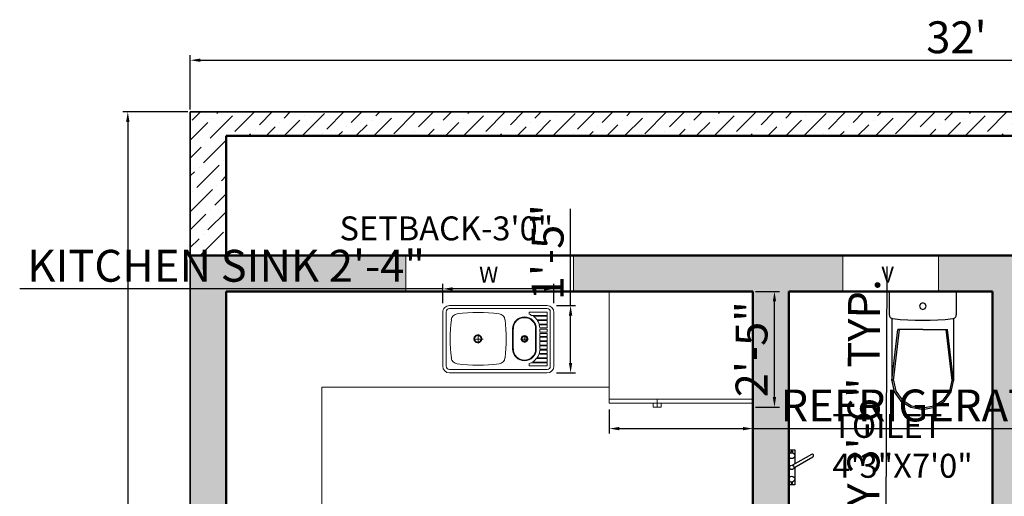
# Model space of a CAD drawing. Units: inches. Extents: x 3354 to 4308, y 1668 to 2317.
# Tile 7 of 11: x 3354 to 3600, y 2198 to 2317. Entities that reach past the tile are written whole.
import ezdxf

# ---------------------------------------------------------------- set-up
doc = ezdxf.new("R2010")
doc.units = ezdxf.units.IN
for name, color, linetype, lineweight in [('A-ANNO-DIMS', 2, 'Continuous', 18), ('A-ANNO-TEXT', 7, 'Continuous', 18), ('A-AREA-IDEN', 3, 'Continuous', 18), ('A-EQPM', 9, 'Continuous', 18), ('A-FLOR-FIXT', 8, 'Continuous', 18), ('A-FURN', 8, 'Continuous', 18), ('A-GLAZ', 4, 'Continuous', 18), ('A-WALL', 7, 'Continuous', 50), ('A-WALL-PATT', 8, 'Continuous', 13), ('C-PROP', 1, 'Continuous', 35)]:
    doc.layers.add(name, color=color, linetype=linetype, lineweight=lineweight)
doc.layers.add('SANTEH', color=7, linetype='Continuous')
doc.styles.get("Standard").update_dxf_attribs({"font": 'arial.ttf'})
doc.dimstyles.new('ISO-25', dxfattribs={"dimtxt": 8, "dimasz": 2.5, "dimexe": 1.25, "dimexo": 0.625, "dimtad": 1, "dimdec": 1, "dimlunit": 3, "dimtxsty": 'Standard', "dimcen": 2.5, "dimadec": 0, "dimazin": 0, "dimtfac": 1, "dimtdec": 1, "dimtmove": 0, "dimatfit": 3, "dimfxl": 1, "dimarcsym": 0})

# ---------------------------------------------------------------- blocks, each defined once
blk = doc.blocks.new('sink 1')
for points in [[(5.86, 24.22), (-5.86, 24.22)], [(-7.34, 1.48), (-7.34, 22.73)], [(-6.56, 1.48), (-6.56, 22.73)], [(6.01, 23.43), (-5.86, 23.43)], [(6.72, 1.48), (6.72, 22.73)], [(7.34, 1.48), (7.34, 22.73)], [(0, 15.39), (0, 17.42)], [(1.09, 16.48), (-0.94, 16.48)], [(-2.09, 8.99), (2.28, 8.99)], [(-2.09, 8.84), (2.28, 8.84)], [(0, 5.55), (0, 7.26)], [(-5.78, 5.39), (-5.78, 5.39)], [(-5.31, 5.39), (-5.31, 5.39)], [(-5.16, 4.92), (-5.16, 4.92)], [(-5, 1.48), (-5, 4.69)], [(-4.84, 4.45), (-4.84, 4.45)], [(0.78, 6.33), (-0.78, 6.33)], [(5, 4.45), (5, 4.45)], [(5.16, 4.92), (5.16, 4.92)], [(5.94, 5.39), (5.94, 5.39)], [(-5, 1.48), (-4.22, 1.48), (-4.22, 3.83)], [(-4.22, 3.83), (-4.22, 3.83)], [(-4.06, 1.48), (-4.06, 3.69)], [(-4.06, 1.48), (-3.28, 1.48), (-3.28, 3.27)], [(-3.91, 3.52), (-3.91, 3.52)], [(-3.28, 3.2), (-3.28, 3.2)], [(-3.12, 3.2), (-3.12, 3.2)], [(-2.34, 3.05), (-2.34, 3.05)], [(-2.19, 3.05), (-2.19, 3.05)], [(-2.09, 3.99), (2.28, 3.99)], [(-2.09, 3.84), (2.28, 3.84)], [(-1.41, 3.05), (-1.41, 3.05)], [(-1.25, 3.05), (-1.25, 3.05)], [(-0.47, 1.48), (-1.25, 1.48), (-1.25, 3.05), (-0.47, 3.05)], [(-0.62, 3.05), (-0.62, 3.05)], [(-0.47, 1.48), (-0.47, 3.05)], [(-0.31, 3.05), (-0.31, 3.05)], [(0.47, 1.48), (-0.31, 1.48), (-0.31, 3.05), (0.47, 3.05)], [(0.31, 3.05), (0.31, 3.05)], [(0.47, 1.48), (0.47, 3.05)], [(0.62, 3.05), (0.62, 3.05)], [(1.25, 3.05), (1.25, 3.05)], [(1.56, 3.05), (1.56, 3.05)], [(2.19, 3.05), (2.19, 3.05)], [(2.5, 3.05), (2.5, 3.05)], [(3.12, 3.2), (3.12, 3.2)], [(3.28, 1.48), (4.06, 1.48), (4.06, 3.57)], [(3.28, 1.48), (3.28, 3.2)], [(3.44, 3.2), (3.44, 3.2)], [(4.06, 3.52), (4.06, 3.52)], [(4.22, 1.48), (4.22, 3.67)], [(4.37, 3.83), (4.37, 3.83)], [(6.01, 0.78), (-5.86, 0.78)], [(5.86, 0), (-5.86, 0)], [(-5.78, 1.48), (-5.78, 1.48)], [(-5.16, 1.48), (-5.16, 1.48)], [(-4.84, 1.48), (-4.84, 1.48)], [(-4.22, 1.48), (-4.22, 1.48)], [(-3.91, 1.48), (-3.91, 1.48)], [(-3.28, 1.48), (-3.28, 1.48)], [(-3.12, 1.48), (-3.12, 1.48)], [(-2.34, 1.48), (-2.34, 1.48)], [(-2.19, 1.48), (-2.19, 1.48)], [(-1.41, 1.48), (-1.41, 1.48)], [(-1.25, 1.48), (-1.25, 1.48)], [(-0.62, 1.48), (-0.62, 1.48)], [(-0.31, 1.48), (-0.31, 1.48)], [(0.31, 1.48), (0.31, 1.48)], [(0.62, 1.48), (0.62, 1.48)], [(1.25, 1.48), (1.25, 1.48)], [(1.56, 1.48), (1.56, 1.48)], [(2.19, 1.48), (2.19, 1.48)], [(2.5, 1.48), (2.5, 1.48)], [(3.12, 1.48), (3.12, 1.48)], [(3.44, 1.48), (3.44, 1.48)], [(4.06, 1.48), (4.06, 1.48)], [(4.37, 1.48), (4.37, 1.48)], [(5, 1.48), (5, 1.48)], [(5.16, 1.48), (5.16, 1.48)], [(5.94, 1.48), (5.94, 1.48)]]:
    blk.add_lwpolyline(points)
for points in [[(-5.16, 4.92), (-5.16, 1.48), (-5.78, 1.48), (-5.78, 5.39), (-5.31, 5.39, -0.068511), (-5.16, 4.92)], [(4.22, 1.48), (5, 1.48), (5, 4.45, -0.083542), (4.22, 3.67, -0.083542)], [(5.16, 4.92, 0.248301), (5.47, 5.39), (5.94, 5.39), (5.94, 1.48), (5.16, 1.48), (5.16, 4.92)], [(4.06, 3.57, -0.061679), (3.32, 3.22)]]:
    blk.add_lwpolyline(points, format="xyb")
for points in [[(-3.12, 3.22), (-3.12, 1.48), (-2.34, 1.48), (-2.34, 3.05, -0.06228)], [(2.5, 3.05), (2.5, 1.48), (3.12, 1.48), (3.12, 3.2, -0.050256)]]:
    blk.add_lwpolyline(points, format="xyb", close=True)
for points in [[(-2.19, 3.05), (-1.41, 3.05), (-1.41, 1.48), (-2.19, 1.48)], [(0.62, 3.05), (1.25, 3.05), (1.25, 1.48), (0.62, 1.48)], [(2.19, 1.48), (2.19, 3.05), (1.56, 3.05), (1.56, 1.48)]]:
    blk.add_lwpolyline(points, close=True)
for centre, radius in [((0.09, 16.57), 0.859), ((0.09, 16.57), 0.703), ((0.09, 6.41), 0.703), ((0.09, 6.41), 0.547)]:
    blk.add_circle(centre, radius)
for centre, radius, start, end in [((-5.86, 22.73), 1.48, 90, 180), ((5.86, 22.73), 1.48, 360, 90), ((-5.86, 22.73), 0.703, 90, 180), ((-3.87, 20.82), 1.53, 97.3256, 171.1849), ((0.09, -12.65), 35.23, 83.2159, 96.7841), ((4.06, 20.82), 1.53, 8.8151, 82.6744), ((6.01, 22.73), 0.703, 0, 90), ((30.19, 16.56), 35.85, 172.7947, 187.4213), ((-30, 16.56), 35.85, 352.5787, 7.2053), ((-3.89, 12.12), 1.48, 187.4212, 263.2159), ((4.08, 12.12), 1.48, 276.7841, 352.5788), ((-2.1, 6.41), 2.58, 90, 270), ((-2.1, 6.41), 2.42, 90, 270), ((0.09, 45.63), 35.23, 263.2159, 276.7841), ((2.28, 6.41), 2.58, 270, 90), ((2.28, 6.41), 2.42, 270, 90), ((-2.15, 6.48), 3.36, 212.1095, 232.0862), ((-2.1, 6.41), 3.36, 234.156, 249.3275), ((2.14, 6.36), 3.36, 289.8633, 290.5971), ((-5.86, 1.48), 1.48, 180, 270), ((-5.86, 1.48), 0.703, 180, 270), ((5.86, 1.48), 1.48, 270, 0), ((6.01, 1.48), 0.703, 270, 360)]:
    blk.add_arc(centre, radius, start, end)
blk = doc.blocks.new('WC 2 Symb_109')
at = {"layer": 'SANTEH'}
for p, q in [((0, 0), (0, 380)), ((0, 380), (132.4, 380)), ((153.6, 364.9), (506.8, 364.9)), ((506.3, 364.9), (215.7, 330.9)), ((506.3, 356), (215.7, 322)), ((215.7, 190), (215.7, 330.9)), ((215.7, 190), (215.7, 49.1)), ((506.3, 24), (215.7, 58)), ((153.8, 15.1), (506.8, 15.1)), ((506.3, 15.1), (215.7, 49.1)), ((0, 0), (132.4, 0))]:
    blk.add_line(p, q, dxfattribs=at)
for points in [[(154.6, 360.1), (153.9, 364.1), (152.3, 367.9), (150.2, 371.3), (147.4, 374.3), (144.1, 376.7), (140.5, 378.5), (136.5, 379.6), (132.4, 380)], [(154.6, 19.7), (158.6, 62.1), (161.4, 104.7), (163.1, 147.3), (163.7, 189.9), (163.1, 232.5), (161.4, 275.1), (158.6, 317.7), (154.6, 360.1)], [(506.3, 24), (565.5, 36.6), (615.7, 72.6), (649.2, 126.5), (661, 190), (649.2, 253.5), (615.7, 307.4), (565.5, 343.4), (506.3, 356)], [(506.8, 15.1), (569.2, 28.4), (622.2, 66.3), (657.6, 123.1), (670, 190), (657.6, 256.9), (622.2, 313.7), (569.2, 351.6), (506.8, 364.9)], [(132.4, 0), (136.5, 0.4), (140.4, 1.5), (144.1, 3.2), (147.3, 5.6), (150.1, 8.6), (152.3, 12), (153.8, 15.7), (154.6, 19.7)]]:
    blk.add_lwpolyline(points, dxfattribs=at)
blk.add_lwpolyline([(83.6, 208.5), (70.4, 203.1), (64.9, 190), (70.4, 176.9), (83.6, 171.5), (96.8, 176.9), (102.2, 190), (96.8, 203.1)], close=True, dxfattribs=at)
blk = doc.blocks.new('Faucet - kit sink top')
at = {"layer": 'SANTEH'}
for p, q in [((-5.5, -0.75), (-5.5, -1.25)), ((-4.94278, -0.75), (-5.5, -0.75)), ((-5.5, -1.25), (-4.94278, -1.25)), ((-0.14775, -1.7441), (3.56698, -8.1782)), ((4.43301, -7.6782), (0.71828, -1.2441)), ((4.94278, -0.75), (5.5, -0.75)), ((5.5, -1.25), (4.94278, -1.25)), ((5.5, -0.75), (5.5, -1.25))]:
    blk.add_line(p, q, dxfattribs=at)
blk.add_lwpolyline([(-0.00587, -2), (-6, -2), (-6, 0), (6, 0), (6, -2), (1.15195, -2)], dxfattribs=at)
for centre, radius in [((-4, -1), 1), ((4, -1), 1), ((0, -1), 0.75)]:
    blk.add_circle(centre, radius, dxfattribs=at)
blk.add_arc((4, -7.9282), 0.5, 210, 30, dxfattribs=at)
blk = doc.blocks.new('Refrigerator-2 door - 36 in top')
for p, q in [((0, -26.999999), (36, -26.999999)), ((12, -26.999999), (12, -28.999999)), ((11, -27.999999), (11, -28.999999)), ((11, -28.999999), (13, -28.999999)), ((13, -28.999999), (13, -27.999999))]:
    blk.add_line(p, q)
blk.add_lwpolyline([(0, -27.999999), (0, 0), (36, 0), (36, -27.999999)], close=True)
blk = doc.blocks.new('*D49')
at = {"layer": 'A-ANNO-DIMS', "color": 0, "lineweight": -2, "transparency": 16777216}
for p, q in [((3396.28, 2294.92), (3396.28, 2308.52)), ((3398.78, 2307.27), (3777.78, 2307.27)), ((3780.28, 2294.92), (3780.28, 2308.52))]:
    blk.add_line(p, q, dxfattribs=at)
at = {"layer": 'A-ANNO-DIMS', "color": 0, "transparency": 16777216}
for points in [[(3398.78, 2307.68), (3398.78, 2306.85), (3396.28, 2307.27)], [(3777.78, 2307.68), (3777.78, 2306.85), (3780.28, 2307.27)]]:
    blk.add_solid(points, dxfattribs=at)
at = {"layer": 'Defpoints', "color": 0, "transparency": 16777216}
for p in [(3780.28, 2307.27), (3396.28, 2294.3), (3780.28, 2294.3)]:
    blk.add_point(p, dxfattribs=at)
at = {"layer": 'A-ANNO-DIMS', "color": 0, "transparency": 16777216, "insert": (3588.28, 2311.98), "char_height": 8, "attachment_point": 5}
blk.add_mtext("32'", dxfattribs=at)
blk = doc.blocks.new('*D50')
at = {"layer": 'A-ANNO-DIMS', "color": 0, "lineweight": -2, "transparency": 16777216}
for p, q in [((3395.65, 2294.3), (3379.37, 2294.3)), ((3380.62, 2291.8), (3380.62, 1756.8)), ((3395.65, 1754.3), (3379.37, 1754.3))]:
    blk.add_line(p, q, dxfattribs=at)
at = {"layer": 'A-ANNO-DIMS', "color": 0, "transparency": 16777216}
for points in [[(3380.2, 2291.8), (3381.04, 2291.8), (3380.62, 2294.3)], [(3380.2, 1756.8), (3381.04, 1756.8), (3380.62, 1754.3)]]:
    blk.add_solid(points, dxfattribs=at)
at = {"layer": 'Defpoints', "color": 0, "transparency": 16777216}
for p in [(3396.28, 2294.3), (3380.62, 1754.3), (3396.28, 1754.3)]:
    blk.add_point(p, dxfattribs=at)
at = {"layer": 'A-ANNO-DIMS', "color": 0, "transparency": 16777216, "insert": (3375.93, 2024.3), "char_height": 8, "attachment_point": 5, "rotation": 90}
blk.add_mtext("45'", dxfattribs=at)
blk = doc.blocks.new('*D68')
at = {"layer": 'A-ANNO-DIMS', "color": 0, "lineweight": -2, "transparency": 16777216}
for p, q in [((3570.57, 2159.15), (3570.89, 2255.55)), ((3564.92, 2159.17), (3571.82, 2159.15)), ((3570.44, 2119.83), (3570.56, 2156.65)), ((3564.78, 2117.35), (3571.68, 2117.33))]:
    blk.add_line(p, q, dxfattribs=at)
at = {"layer": 'A-ANNO-DIMS', "color": 0, "transparency": 16777216}
for points in [[(3570.14, 2156.65), (3570.98, 2156.65), (3570.57, 2159.15)], [(3570.02, 2119.83), (3570.85, 2119.83), (3570.43, 2117.33)]]:
    blk.add_solid(points, dxfattribs=at)
at = {"layer": 'Defpoints', "color": 0, "transparency": 16777216}
for p in [(3564.29, 2159.17), (3570.57, 2159.15), (3564.15, 2117.35)]:
    blk.add_point(p, dxfattribs=at)
at = {"layer": 'A-ANNO-DIMS', "color": 0, "transparency": 16777216, "insert": (3566.02, 2208.62), "char_height": 8, "attachment_point": 5, "rotation": 89.8084}
blk.add_mtext('VANITY 3\'-6" TYP.', dxfattribs=at)
blk = doc.blocks.new('*D80')
at = {"layer": 'A-ANNO-DIMS', "color": 0, "lineweight": -2, "transparency": 16777216}
for p, q in [((3459.54, 2246.37), (3459.54, 2251.18)), ((3487.4, 2246.37), (3487.4, 2251.18)), ((3459.54, 2249.93), (3353.53, 2249.93)), ((3484.9, 2249.93), (3462.04, 2249.93))]:
    blk.add_line(p, q, dxfattribs=at)
at = {"layer": 'A-ANNO-DIMS', "color": 0, "transparency": 16777216}
for points in [[(3462.04, 2250.34), (3462.04, 2249.51), (3459.54, 2249.93)], [(3484.9, 2250.34), (3484.9, 2249.51), (3487.4, 2249.93)]]:
    blk.add_solid(points, dxfattribs=at)
at = {"layer": 'Defpoints', "color": 0, "transparency": 16777216}
for p in [(3459.54, 2249.93), (3459.54, 2245.75), (3487.4, 2245.75)]:
    blk.add_point(p, dxfattribs=at)
at = {"layer": 'A-ANNO-DIMS', "color": 0, "transparency": 16777216, "insert": (3405.28, 2254.69), "char_height": 8, "attachment_point": 5}
blk.add_mtext('KITCHEN SINK 2\'-4"', dxfattribs=at)
blk = doc.blocks.new('*D81')
at = {"layer": 'A-ANNO-DIMS', "color": 0, "lineweight": -2, "transparency": 16777216}
for p, q in [((3491.58, 2245.75), (3491.58, 2270.01)), ((3488.03, 2245.75), (3492.83, 2245.75)), ((3491.58, 2231.35), (3491.58, 2243.25)), ((3488.03, 2228.85), (3492.83, 2228.85))]:
    blk.add_line(p, q, dxfattribs=at)
at = {"layer": 'A-ANNO-DIMS', "color": 0, "transparency": 16777216}
for points in [[(3491.17, 2243.25), (3492, 2243.25), (3491.58, 2245.75)], [(3491.17, 2231.35), (3492, 2231.35), (3491.58, 2228.85)]]:
    blk.add_solid(points, dxfattribs=at)
at = {"layer": 'Defpoints', "color": 0, "transparency": 16777216}
for p in [(3487.4, 2245.75), (3491.58, 2245.75), (3487.4, 2228.85)]:
    blk.add_point(p, dxfattribs=at)
at = {"layer": 'A-ANNO-DIMS', "color": 0, "transparency": 16777216, "insert": (3486.87, 2259.13), "char_height": 8, "attachment_point": 5, "rotation": 90}
blk.add_mtext('1\'-5"', dxfattribs=at)
blk = doc.blocks.new('*D84')
at = {"layer": 'A-ANNO-DIMS', "color": 0, "lineweight": -2, "transparency": 16777216}
for p, q in [((3501.28, 2219.67), (3501.28, 2213.65)), ((3537.28, 2219.67), (3537.28, 2213.65)), ((3503.78, 2214.9), (3534.78, 2214.9)), ((3537.28, 2214.9), (3653.77, 2214.9))]:
    blk.add_line(p, q, dxfattribs=at)
at = {"layer": 'A-ANNO-DIMS', "color": 0, "transparency": 16777216}
for points in [[(3503.78, 2215.31), (3503.78, 2214.48), (3501.28, 2214.9)], [(3534.78, 2215.31), (3534.78, 2214.48), (3537.28, 2214.9)]]:
    blk.add_solid(points, dxfattribs=at)
at = {"layer": 'Defpoints', "color": 0, "transparency": 16777216}
for p in [(3501.28, 2220.3), (3537.28, 2220.3), (3537.28, 2214.9)]:
    blk.add_point(p, dxfattribs=at)
at = {"layer": 'A-ANNO-DIMS', "color": 0, "transparency": 16777216, "insert": (3596.78, 2219.66), "char_height": 8, "attachment_point": 5}
blk.add_mtext('REFRIGERATOR 3\'-0"', dxfattribs=at)
blk = doc.blocks.new('*D85')
at = {"layer": 'A-ANNO-DIMS', "color": 0, "lineweight": -2, "transparency": 16777216}
for p, q in [((3537.9, 2249.3), (3543.93, 2249.3)), ((3542.68, 2222.8), (3542.68, 2246.8)), ((3537.9, 2220.3), (3543.93, 2220.3))]:
    blk.add_line(p, q, dxfattribs=at)
at = {"layer": 'A-ANNO-DIMS', "color": 0, "transparency": 16777216}
for points in [[(3542.26, 2246.8), (3543.09, 2246.8), (3542.68, 2249.3)], [(3542.26, 2222.8), (3543.09, 2222.8), (3542.68, 2220.3)]]:
    blk.add_solid(points, dxfattribs=at)
at = {"layer": 'Defpoints', "color": 0, "transparency": 16777216}
for p in [(3537.28, 2249.3), (3542.68, 2249.3), (3537.28, 2220.3)]:
    blk.add_point(p, dxfattribs=at)
at = {"layer": 'A-ANNO-DIMS', "color": 0, "transparency": 16777216, "insert": (3537.97, 2234.8), "char_height": 8, "attachment_point": 5, "rotation": 90}
blk.add_mtext('2\'-5"', dxfattribs=at)

msp = doc.modelspace()

# ---------------------------------------------------------------- hatches: boundary and pattern name
at = {"layer": 'A-WALL-PATT', "transparency": 33554687}
h = msp.add_hatch(dxfattribs=at)
h.set_pattern_fill('ANSI36', color=256)
h.paths.add_polyline_path([(3780.28, 2294.3), (3396.28, 2294.3), (3396.28, 2258.3), (3405.28, 2258.3), (3405.28, 2288.3), (3780.28, 2288.3)])
h = msp.add_hatch(color=256, dxfattribs=at)
h.dxf.hatch_style = 1
h.paths.add_polyline_path([(3546.28, 1829.3), (3552.28, 1829.3), (3552.28, 1838.3), (3546.28, 1838.3), (3546.28, 1910.3), (3582.28, 1910.3), (3582.28, 1919.3), (3546.28, 1919.3), (3546.28, 1961.3), (3534.28, 1961.3), (3534.28, 1955.3), (3537.28, 1955.3), (3537.28, 1808.3), (3516.28, 1808.3), (3516.28, 1799.3), (3546.28, 1799.3)])
h.paths.add_polyline_path([(3672.28, 1919.3), (3656.51, 1919.3), (3630.28, 1919.3), (3630.28, 1910.3), (3642.28, 1910.3), (3642.28, 1838.3), (3630.28, 1838.3), (3630.28, 1835.3), (3630.28, 1829.3), (3642.28, 1829.3), (3642.28, 1799.3), (3651.28, 1799.3), (3651.28, 1910.3), (3672.28, 1910.3)])
h.paths.add_polyline_path([(3744.28, 1959.8), (3735.28, 1959.8), (3735.28, 1923.23), (3735.28, 1919.3), (3714.28, 1919.3), (3714.28, 1910.3), (3744.28, 1910.3)])
h.paths.add_polyline_path([(3744.28, 2072.3), (3735.28, 2072.3), (3735.28, 2031.8), (3744.28, 2031.8)])
h.paths.add_polyline_path([(3744.28, 2150.3), (3735.28, 2150.3), (3735.28, 2108.3), (3744.28, 2108.3)])
h.paths.add_polyline_path([(3744.28, 2258.3), (3705.28, 2258.3), (3705.28, 2249.3), (3735.28, 2249.3), (3735.28, 2210.3), (3744.28, 2210.3)])
h.paths.add_polyline_path([(3633.28, 2258.3), (3583.78, 2258.3), (3583.78, 2249.3), (3588.24, 2249.3), (3597.28, 2249.3), (3597.28, 2165.3), (3594.28, 2165.3), (3594.28, 2159.3), (3597.28, 2159.3), (3597.28, 2117.3), (3594.28, 2117.3), (3594.28, 2111.3), (3603.28, 2111.3), (3603.28, 2249.3), (3633.28, 2249.3)])
h.paths.add_polyline_path([(3559.78, 2258.3), (3492.28, 2258.3), (3492.28, 2249.3), (3537.28, 2249.3), (3537.28, 2117.3), (3534.28, 2117.3), (3534.28, 2111.3), (3564.28, 2111.3), (3564.28, 2117.3), (3546.28, 2117.3), (3546.28, 2159.3), (3564.28, 2159.3), (3564.28, 2165.3), (3546.28, 2165.3), (3546.28, 2249.3), (3559.78, 2249.3)])
h.paths.add_polyline_path([(3450.28, 2258.3), (3396.28, 2258.3), (3396.28, 1799.3), (3474.28, 1799.3), (3474.28, 1808.3), (3405.28, 1808.3), (3405.28, 1955.3), (3498.28, 1955.3), (3498.28, 1961.3), (3405.28, 1961.3), (3405.28, 2111.3), (3498.28, 2111.3), (3498.28, 2117.3), (3405.28, 2117.3), (3405.28, 2249.3), (3450.28, 2249.3)])
h.paths.add_polyline_path([(3582.28, 1838.3), (3576.28, 1838.3), (3576.28, 1829.3), (3582.28, 1829.3)], flags=17)

# ---------------------------------------------------------------- linework, layer by layer
at = {"layer": 'A-FURN'}
for p, q in [((3501.28, 2249.3), (3501.28, 2225.3)), ((3429.28, 2225.3), (3429.28, 2117.3)), ((3501.28, 2225.3), (3429.28, 2225.3))]:
    msp.add_line(p, q, dxfattribs=at)
at = {"layer": 'A-GLAZ'}
for p, q in [((3450.28, 2249.3), (3450.28, 2258.3)), ((3492.28, 2249.3), (3492.28, 2258.3)), ((3559.78, 2249.3), (3559.78, 2258.3)), ((3583.78, 2249.3), (3583.78, 2258.3))]:
    msp.add_line(p, q, dxfattribs=at)
at = {"layer": 'A-WALL'}
for p, q in [((3405.28, 2258.3), (3405.28, 2288.3)), ((3405.28, 2288.3), (3780.28, 2288.3)), ((3744.28, 2258.3), (3396.28, 2258.3)), ((3405.28, 2249.3), (3405.28, 2117.3)), ((3537.28, 2249.3), (3405.28, 2249.3)), ((3537.28, 2249.3), (3537.28, 2117.3)), ((3546.28, 2249.3), (3546.28, 2165.3)), ((3597.28, 2249.3), (3546.28, 2249.3)), ((3597.28, 2165.3), (3597.28, 2249.3))]:
    msp.add_line(p, q, dxfattribs=at)
at = {"layer": 'C-PROP'}
msp.add_lwpolyline([(3738.28, 1754.3), (3780.28, 1754.3), (3780.28, 2294.3), (3396.28, 2294.3), (3396.28, 1754.3), (3576.28, 1754.3)], dxfattribs=at)

# ---------------------------------------------------------------- block references
at = {"layer": 'A-EQPM'}
msp.add_blockref('Refrigerator-2 door - 36 in top', (3501.28, 2249.3), dxfattribs=at)
at = {"layer": 'A-FLOR-FIXT'}
for name, p, xscale, yscale, zscale, rotation in [('WC 2 Symb_109', (3571.45, 2249.3), 0.0441898926459964, 0.0441898926459964, 0.0441898926459964, 269.9999999999999), ('sink 1', (3487.4, 2237.3), 1.150769176553845, 1.150769176553845, 1.150769176553845, 90), ('Faucet - kit sink top', (3546.28, 2205.18), 0.7356136897818673, 0.7356136897818673, 0.7356136897818673, 90)]:
    msp.add_blockref(name, p, dxfattribs=dict(at, xscale=xscale, yscale=yscale, zscale=zscale, rotation=rotation))

# ---------------------------------------------------------------- texts
at = {"layer": 'A-ANNO-TEXT', "attachment_point": 1}
for s, width, insert, char_height in [('{SETBACK-3\'0"}', 74.5832, (3433.67, 2268.1), 6), ('\\pxt6;{W}', 32.7844, (3468.66, 2255.52), 4), ('\\pxt6;{V}', 32.7844, (3569.48, 2255.52), 4)]:
    msp.add_mtext_dynamic_manual_height_columns(s, width=width, gutter_width=12.5, heights=[0], dxfattribs=dict(at, insert=insert, char_height=char_height))
at = {"layer": 'A-AREA-IDEN', "insert": (3557.19, 2218.58), "char_height": 6, "attachment_point": 1}
msp.add_mtext_dynamic_manual_height_columns('TOILET\\P4\'3"X7\'0"', width=74.5832, gutter_width=12.5, heights=[0], dxfattribs=at)

# ---------------------------------------------------------------- dimensions: what is measured, and where the dimension line sits
at = {"layer": 'A-ANNO-DIMS'}
dim = msp.add_linear_dim(base=(3780.28, 2307.27), p1=(3396.28, 2294.3), p2=(3780.28, 2294.3), dimstyle='ISO-25', override={"dimclrd": 0, "dimclre": 0, "dimclrt": 0}, dxfattribs=at)
dim.commit()
dim.dimension.update_dxf_attribs({"geometry": '*D49', "text_midpoint": (3588.28, 2311.98)})
for base, p1, p2, override, picture, middle in [((3380.62, 1754.3), (3396.28, 2294.3), (3396.28, 1754.3), {"dimclrd": 0, "dimclre": 0, "dimclrt": 0}, '*D50', (3375.93, 2024.3)), ((3491.58, 2245.75), (3487.4, 2228.85), (3487.4, 2245.75), {"dimdec": 1, "dimrnd": 0, "dimzin": 1, "dimlunit": 4, "dimfrac": 2}, '*D81', (3486.87, 2259.13)), ((3542.68, 2249.3), (3537.28, 2220.3), (3537.28, 2249.3), {"dimdec": 1, "dimrnd": 0, "dimzin": 1, "dimlunit": 4, "dimfrac": 2}, '*D85', (3537.97, 2234.8))]:
    dim = msp.add_linear_dim(base=base, p1=p1, p2=p2, angle=90, dimstyle='ISO-25', override=override, dxfattribs=at)
    dim.commit()
    dim.dimension.update_dxf_attribs({"geometry": picture, "text_midpoint": middle})
for base, p1, p2, angle, text, picture, middle in [((3459.54, 2249.93), (3487.4, 2245.75), (3459.54, 2245.75), 180, 'KITCHEN SINK <>', '*D80', (3405.28, 2254.69)), ((3570.57, 2159.15), (3564.15, 2117.35), (3564.29, 2159.17), 89.8084, 'VANITY <> TYP.', '*D68', (3566.02, 2208.62))]:
    dim = msp.add_linear_dim(base=base, p1=p1, p2=p2, angle=angle, text=text, dimstyle='ISO-25', override={"dimdec": 1, "dimrnd": 0, "dimzin": 1, "dimlunit": 4, "dimfrac": 2}, dxfattribs=at)
    dim.commit()
    dim.dimension.update_dxf_attribs({"geometry": picture, "text_midpoint": middle})
dim = msp.add_linear_dim(base=(3537.28, 2214.9), p1=(3501.28, 2220.3), p2=(3537.28, 2220.3), text='REFRIGERATOR <>', dimstyle='ISO-25', override={"dimdec": 1, "dimrnd": 0, "dimzin": 1, "dimlunit": 4, "dimfrac": 2}, dxfattribs=at)
dim.commit()
dim.dimension.update_dxf_attribs({"geometry": '*D84', "text_midpoint": (3596.78, 2219.66)})

doc.saveas('drawing.dxf')
